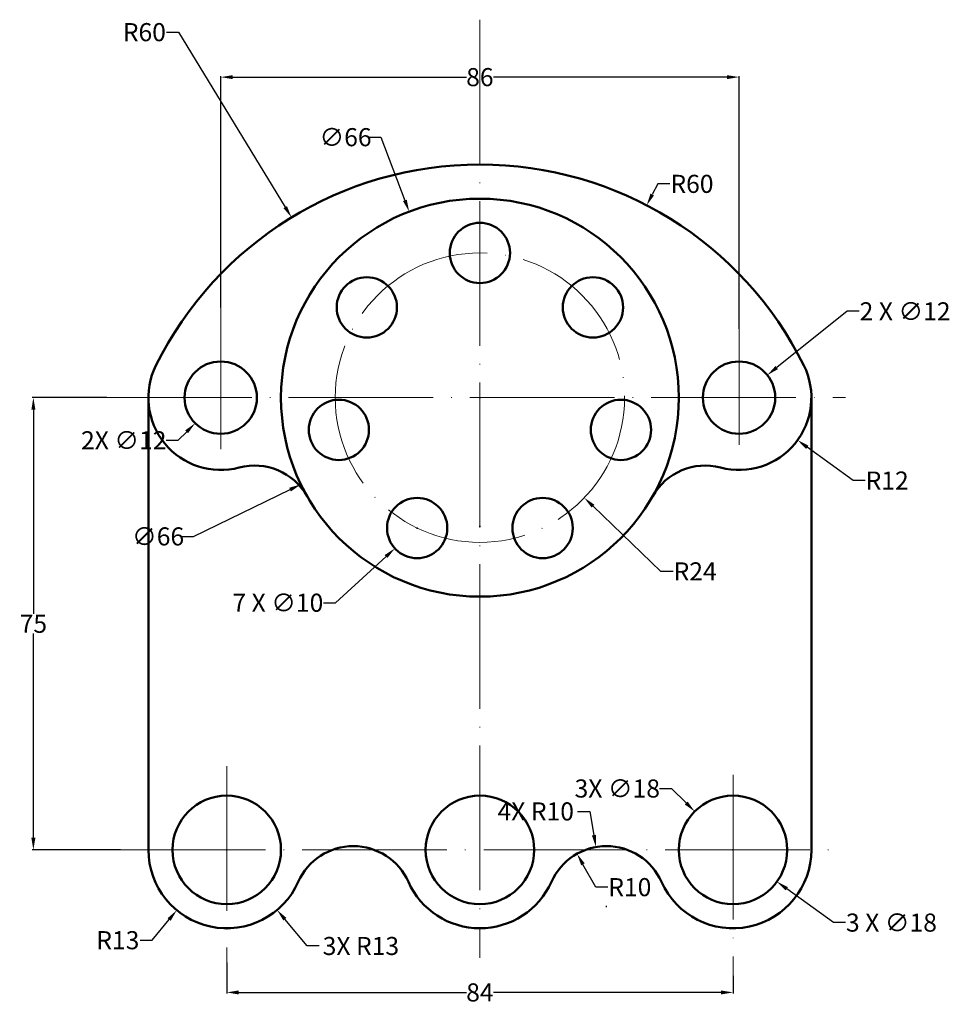
# Model space of a CAD drawing. Units: inches. Extents: x 328 to 483, y 163 to 326.
import ezdxf

# ---------------------------------------------------------------- set-up
doc = ezdxf.new("R2010")
doc.units = ezdxf.units.IN
doc.header["$MEASUREMENT"] = 0
doc.linetypes.add('ACAD_ISO04W100', pattern=[30, 24, -3, 0, -3])
for name, color, linetype, lineweight in [('M-CNTR', 4, 'ACAD_ISO04W100', 18), ('M-DIMS', 2, 'Continuous', 25), ('M-OUTL', 7, 'Continuous', 50)]:
    doc.layers.add(name, color=color, linetype=linetype, lineweight=lineweight)
doc.styles.get("Standard").update_dxf_attribs({"font": 'arial.ttf'})
doc.dimstyles.get("Standard").update_dxf_attribs({"dimtxt": 3, "dimasz": 2, "dimexe": 0.18, "dimexo": 0.0625, "dimgap": 0.09, "dimtad": 0, "dimtih": 1, "dimtoh": 1, "dimdec": 0, "dimzin": 0, "dimdsep": 46, "dimtxsty": 'Standard', "dimcen": 0.09, "dimclrd": 1, "dimclre": 1, "dimadec": 0, "dimazin": 0, "dimtfac": 1, "dimtdec": 0, "dimtofl": 0, "dimtmove": 0, "dimatfit": 3, "dimfxl": 1, "dimtolj": 1, "dimtzin": 0, "dimarcsym": 0})

# ---------------------------------------------------------------- blocks, each defined once
blk = doc.blocks.new('*U1')
blk.add_circle((0, 0), 5)
blk = doc.blocks.new('*U2')
at = {"layer": 'M-OUTL', "color": 0, "linetype": 'ByBlock', "lineweight": -2, "transparency": 16777216}
blk.add_blockref('*U1', (404.65, 287.76), dxfattribs=at)
for p, rotation in [((385.89, 278.73), 51.42857142857143), ((423.41, 278.73), 308.5714285714285), ((381.25, 258.42), 102.8571428571428), ((428.05, 258.42), 257.1428571428572), ((394.24, 242.14), 154.2857142857143), ((415.06, 242.14), 205.7142857142856)]:
    blk.add_blockref('*U1', p, dxfattribs=dict(at, rotation=rotation))
blk = doc.blocks.new('*D3')
at = {"layer": 'Defpoints', "color": 0, "transparency": 16777216}
for p in [(439.36, 194.04), (453.94, 183.49)]:
    blk.add_point(p, dxfattribs=at)
at = {"layer": 'M-DIMS', "color": 0, "lineweight": -2, "transparency": 16777216}
for p, q in [((446.56, 188.76), (446.74, 188.76)), ((446.65, 188.67), (446.65, 188.85)), ((463.34, 176.7), (455.57, 182.32)), ((465.34, 176.7), (463.34, 176.7))]:
    blk.add_line(p, q, dxfattribs=at)
at = {"layer": 'M-DIMS', "color": 0, "transparency": 16777216}
blk.add_solid([(455.76, 182.59), (455.37, 182.05), (453.94, 183.49)], dxfattribs=at)
at = {"layer": 'M-DIMS', "color": 0, "transparency": 16777216, "insert": (472.94, 176.7), "char_height": 3, "attachment_point": 5}
blk.add_mtext('\\A1;3 X ∅18', dxfattribs=at)
blk = doc.blocks.new('*D4')
at = {"layer": 'Defpoints', "color": 0, "transparency": 16777216}
for p in [(420.77, 188.11), (425.65, 179.38)]:
    blk.add_point(p, dxfattribs=at)
at = {"layer": 'M-DIMS', "color": 0, "lineweight": -2, "transparency": 16777216}
for p, q in [((423.87, 182.58), (421.75, 186.36)), ((425.87, 182.58), (423.87, 182.58))]:
    blk.add_line(p, q, dxfattribs=at)
at = {"layer": 'M-DIMS', "color": 0, "transparency": 16777216}
blk.add_solid([(422.04, 186.53), (421.46, 186.2), (420.77, 188.11)], dxfattribs=at)
at = {"layer": 'M-DIMS', "color": 0, "transparency": 16777216, "insert": (429.53, 182.58), "char_height": 3, "attachment_point": 5}
blk.add_mtext('\\A1;R10', dxfattribs=at)
blk = doc.blocks.new('*D5')
at = {"layer": 'Defpoints', "color": 0, "transparency": 16777216}
for p in [(362.65, 170.14), (446.65, 167.94), (446.65, 165.12)]:
    blk.add_point(p, dxfattribs=at)
at = {"layer": 'M-DIMS', "color": 0, "lineweight": -2, "transparency": 16777216}
for p, q in [((362.65, 170.08), (362.65, 164.94)), ((446.65, 167.88), (446.65, 164.94)), ((364.65, 165.12), (402.42, 165.12)), ((444.65, 165.12), (406.89, 165.12))]:
    blk.add_line(p, q, dxfattribs=at)
at = {"layer": 'M-DIMS', "color": 0, "transparency": 16777216}
for points in [[(364.65, 165.45), (364.65, 164.78), (362.65, 165.12)], [(444.65, 165.45), (444.65, 164.78), (446.65, 165.12)]]:
    blk.add_solid(points, dxfattribs=at)
at = {"layer": 'M-DIMS', "color": 0, "transparency": 16777216, "insert": (404.65, 165.12), "char_height": 3, "attachment_point": 5}
blk.add_mtext('\\A1;84', dxfattribs=at)
blk = doc.blocks.new('*D6')
at = {"layer": 'Defpoints', "color": 0, "transparency": 16777216}
for p in [(362.65, 188.76), (354.36, 178.75)]:
    blk.add_point(p, dxfattribs=at)
at = {"layer": 'M-DIMS', "color": 0, "lineweight": -2, "transparency": 16777216}
for p, q in [((362.56, 188.76), (362.74, 188.76)), ((362.65, 188.67), (362.65, 188.85)), ((350.26, 173.78), (353.09, 177.21)), ((348.26, 173.78), (350.26, 173.78))]:
    blk.add_line(p, q, dxfattribs=at)
at = {"layer": 'M-DIMS', "color": 0, "transparency": 16777216}
blk.add_solid([(352.83, 177.42), (353.34, 176.99), (354.36, 178.75)], dxfattribs=at)
at = {"layer": 'M-DIMS', "color": 0, "transparency": 16777216, "insert": (344.58, 173.78), "char_height": 3, "attachment_point": 5}
blk.add_mtext('\\A1;R13', dxfattribs=at)
blk = doc.blocks.new('*D7')
at = {"layer": 'Defpoints', "color": 0, "transparency": 16777216}
for p in [(342.79, 263.76), (330.56, 188.76), (345.08, 188.76)]:
    blk.add_point(p, dxfattribs=at)
at = {"layer": 'M-DIMS', "color": 0, "lineweight": -2, "transparency": 16777216}
for p, q in [((342.73, 263.76), (330.38, 263.76)), ((330.56, 261.76), (330.56, 227.88)), ((330.56, 190.76), (330.56, 224.65)), ((345.02, 188.76), (330.38, 188.76))]:
    blk.add_line(p, q, dxfattribs=at)
at = {"layer": 'M-DIMS', "color": 0, "transparency": 16777216}
for points in [[(330.23, 261.76), (330.9, 261.76), (330.56, 263.76)], [(330.23, 190.76), (330.9, 190.76), (330.56, 188.76)]]:
    blk.add_solid(points, dxfattribs=at)
at = {"layer": 'M-DIMS', "color": 0, "transparency": 16777216, "insert": (330.56, 226.26), "char_height": 3, "attachment_point": 5}
blk.add_mtext('\\A1;75', dxfattribs=at)
blk = doc.blocks.new('*D8')
at = {"layer": 'Defpoints', "color": 0, "transparency": 16777216}
for p in [(447.65, 263.76), (457.36, 256.71)]:
    blk.add_point(p, dxfattribs=at)
at = {"layer": 'M-DIMS', "color": 0, "lineweight": -2, "transparency": 16777216}
for p, q in [((447.56, 263.76), (447.74, 263.76)), ((447.65, 263.67), (447.65, 263.85)), ((466.57, 250.01), (458.97, 255.53)), ((468.57, 250.01), (466.57, 250.01))]:
    blk.add_line(p, q, dxfattribs=at)
at = {"layer": 'M-DIMS', "color": 0, "transparency": 16777216}
blk.add_solid([(459.17, 255.8), (458.78, 255.26), (457.36, 256.71)], dxfattribs=at)
at = {"layer": 'M-DIMS', "color": 0, "transparency": 16777216, "insert": (472.23, 250.01), "char_height": 3, "attachment_point": 5}
blk.add_mtext('\\A1;R12', dxfattribs=at)
blk = doc.blocks.new('*D9')
at = {"layer": 'Defpoints', "color": 0, "transparency": 16777216}
for p in [(404.65, 263.76), (421.97, 247.15)]:
    blk.add_point(p, dxfattribs=at)
at = {"layer": 'M-DIMS', "color": 0, "lineweight": -2, "transparency": 16777216}
for p, q in [((404.56, 263.76), (404.74, 263.76)), ((404.65, 263.67), (404.65, 263.85)), ((434.7, 234.95), (423.42, 245.77)), ((436.7, 234.95), (434.7, 234.95))]:
    blk.add_line(p, q, dxfattribs=at)
at = {"layer": 'M-DIMS', "color": 0, "transparency": 16777216}
blk.add_solid([(423.65, 246.01), (423.19, 245.53), (421.97, 247.15)], dxfattribs=at)
at = {"layer": 'M-DIMS', "color": 0, "transparency": 16777216, "insert": (440.37, 234.95), "char_height": 3, "attachment_point": 5}
blk.add_mtext('\\A1;R24', dxfattribs=at)
blk = doc.blocks.new('*D10')
at = {"layer": 'Defpoints', "color": 0, "transparency": 16777216}
for p in [(397.92, 245.52), (390.55, 238.76)]:
    blk.add_point(p, dxfattribs=at)
at = {"layer": 'M-DIMS', "color": 0, "lineweight": -2, "transparency": 16777216}
for p, q in [((394.15, 242.14), (394.33, 242.14)), ((394.24, 242.05), (394.24, 242.23)), ((380.71, 229.75), (389.08, 237.41)), ((378.71, 229.75), (380.71, 229.75))]:
    blk.add_line(p, q, dxfattribs=at)
at = {"layer": 'M-DIMS', "color": 0, "transparency": 16777216}
blk.add_solid([(388.85, 237.66), (389.3, 237.17), (390.55, 238.76)], dxfattribs=at)
at = {"layer": 'M-DIMS', "color": 0, "transparency": 16777216, "insert": (371.13, 229.75), "char_height": 3, "attachment_point": 5}
blk.add_mtext('\\A1;7 X ∅10', dxfattribs=at)
blk = doc.blocks.new('*D11')
at = {"layer": 'Defpoints', "color": 0, "transparency": 16777216}
for p in [(432.33, 295.67), (404.65, 242.43)]:
    blk.add_point(p, dxfattribs=at)
at = {"layer": 'M-DIMS', "color": 0, "lineweight": -2, "transparency": 16777216}
for p, q in [((434.17, 299.22), (433.25, 297.44)), ((436.17, 299.22), (434.17, 299.22)), ((404.56, 242.43), (404.74, 242.43)), ((404.65, 242.34), (404.65, 242.52))]:
    blk.add_line(p, q, dxfattribs=at)
at = {"layer": 'M-DIMS', "color": 0, "transparency": 16777216}
blk.add_solid([(432.95, 297.6), (433.54, 297.29), (432.33, 295.67)], dxfattribs=at)
at = {"layer": 'M-DIMS', "color": 0, "transparency": 16777216, "insert": (439.84, 299.22), "char_height": 3, "attachment_point": 5}
blk.add_mtext('\\A1;R60', dxfattribs=at)
blk = doc.blocks.new('*D12')
at = {"layer": 'Defpoints', "color": 0, "transparency": 16777216}
for p in [(447.65, 316.92), (361.65, 278.66), (447.65, 275.13)]:
    blk.add_point(p, dxfattribs=at)
at = {"layer": 'M-DIMS', "color": 0, "lineweight": -2, "transparency": 16777216}
for p, q in [((361.65, 278.72), (361.65, 317.1)), ((363.65, 316.92), (402.41, 316.92)), ((445.65, 316.92), (406.89, 316.92)), ((447.65, 275.19), (447.65, 317.1))]:
    blk.add_line(p, q, dxfattribs=at)
at = {"layer": 'M-DIMS', "color": 0, "transparency": 16777216}
for points in [[(363.65, 317.25), (363.65, 316.59), (361.65, 316.92)], [(445.65, 317.25), (445.65, 316.59), (447.65, 316.92)]]:
    blk.add_solid(points, dxfattribs=at)
at = {"layer": 'M-DIMS', "color": 0, "transparency": 16777216, "insert": (404.65, 316.92), "char_height": 3, "attachment_point": 5}
blk.add_mtext('\\A1;86', dxfattribs=at)
blk = doc.blocks.new('*D13')
at = {"layer": 'Defpoints', "color": 0, "transparency": 16777216}
for p in [(452.34, 267.5), (442.96, 260.02)]:
    blk.add_point(p, dxfattribs=at)
at = {"layer": 'M-DIMS', "color": 0, "lineweight": -2, "transparency": 16777216}
for p, q in [((465.59, 278.08), (453.9, 268.75)), ((467.59, 278.08), (465.59, 278.08)), ((447.56, 263.76), (447.74, 263.76)), ((447.65, 263.67), (447.65, 263.85))]:
    blk.add_line(p, q, dxfattribs=at)
at = {"layer": 'M-DIMS', "color": 0, "transparency": 16777216}
blk.add_solid([(453.7, 269.01), (454.11, 268.49), (452.34, 267.5)], dxfattribs=at)
at = {"layer": 'M-DIMS', "color": 0, "transparency": 16777216, "insert": (475.2, 278.08), "char_height": 3, "attachment_point": 5}
blk.add_mtext('\\A1;2 X ∅12', dxfattribs=at)
blk = doc.blocks.new('*D14')
at = {"layer": 'Defpoints', "color": 0, "transparency": 16777216}
for p in [(392.92, 294.61), (416.38, 232.92)]:
    blk.add_point(p, dxfattribs=at)
at = {"layer": 'M-DIMS', "color": 0, "lineweight": -2, "transparency": 16777216}
for p, q in [((386.23, 306.96), (388.23, 306.96)), ((388.23, 306.96), (392.21, 296.48)), ((404.56, 263.76), (404.74, 263.76)), ((404.65, 263.67), (404.65, 263.85))]:
    blk.add_line(p, q, dxfattribs=at)
at = {"layer": 'M-DIMS', "color": 0, "transparency": 16777216}
blk.add_solid([(392.52, 296.6), (391.9, 296.36), (392.92, 294.61)], dxfattribs=at)
at = {"layer": 'M-DIMS', "color": 0, "transparency": 16777216, "insert": (382.36, 306.96), "char_height": 3, "attachment_point": 5}
blk.add_mtext('\\A1;∅66', dxfattribs=at)
blk = doc.blocks.new('*D15')
at = {"layer": 'Defpoints', "color": 0, "transparency": 16777216}
for p in [(373.4, 293.65), (404.65, 242.43)]:
    blk.add_point(p, dxfattribs=at)
at = {"layer": 'M-DIMS', "color": 1, "lineweight": -2, "transparency": 16777216}
for p, q in [((352.65, 324.38), (354.65, 324.38)), ((354.65, 324.38), (372.36, 295.36)), ((404.56, 242.43), (404.74, 242.43)), ((404.65, 242.34), (404.65, 242.52))]:
    blk.add_line(p, q, dxfattribs=at)
at = {"layer": 'M-DIMS', "color": 1, "transparency": 16777216}
blk.add_solid([(372.64, 295.53), (372.07, 295.18), (373.4, 293.65)], dxfattribs=at)
at = {"layer": 'M-DIMS', "color": 0, "transparency": 16777216, "insert": (348.98, 324.38), "char_height": 3, "attachment_point": 5}
blk.add_mtext('\\A1;R60', dxfattribs=at)
blk = doc.blocks.new('*D16')
at = {"layer": 'Defpoints', "color": 0, "transparency": 16777216}
for p in [(434.35, 278.15), (374.95, 249.38)]:
    blk.add_point(p, dxfattribs=at)
at = {"layer": 'M-DIMS', "color": 1, "lineweight": -2, "transparency": 16777216}
for p, q in [((404.56, 263.76), (404.74, 263.76)), ((404.65, 263.67), (404.65, 263.85)), ((357.13, 240.75), (373.15, 248.51)), ((355.13, 240.75), (357.13, 240.75))]:
    blk.add_line(p, q, dxfattribs=at)
at = {"layer": 'M-DIMS', "color": 1, "transparency": 16777216}
blk.add_solid([(373.01, 248.81), (373.3, 248.21), (374.95, 249.38)], dxfattribs=at)
at = {"layer": 'M-DIMS', "color": 0, "transparency": 16777216, "insert": (351.26, 240.75), "char_height": 3, "attachment_point": 5}
blk.add_mtext('\\A1;∅66', dxfattribs=at)
blk = doc.blocks.new('*D17')
at = {"layer": 'Defpoints', "color": 0, "transparency": 16777216}
for p in [(365.89, 268.01), (357.41, 259.52)]:
    blk.add_point(p, dxfattribs=at)
at = {"layer": 'M-DIMS', "color": 1, "lineweight": -2, "transparency": 16777216}
for p, q in [((361.56, 263.76), (361.74, 263.76)), ((361.65, 263.67), (361.65, 263.85)), ((354.58, 256.69), (356, 258.1)), ((352.58, 256.69), (354.58, 256.69))]:
    blk.add_line(p, q, dxfattribs=at)
at = {"layer": 'M-DIMS', "color": 1, "transparency": 16777216}
blk.add_solid([(355.76, 258.34), (356.23, 257.87), (357.41, 259.52)], dxfattribs=at)
at = {"layer": 'M-DIMS', "color": 0, "transparency": 16777216, "insert": (345.56, 256.69), "char_height": 3, "attachment_point": 5}
blk.add_mtext('\\A1;2X ∅12', dxfattribs=at)
blk = doc.blocks.new('*D18')
at = {"layer": 'Defpoints', "color": 0, "transparency": 16777216}
for p in [(362.65, 188.76), (371, 178.8)]:
    blk.add_point(p, dxfattribs=at)
at = {"layer": 'M-DIMS', "color": 1, "lineweight": -2, "transparency": 16777216}
for p, q in [((362.56, 188.76), (362.74, 188.76)), ((362.65, 188.67), (362.65, 188.85)), ((376.01, 172.82), (372.29, 177.27)), ((378.01, 172.82), (376.01, 172.82))]:
    blk.add_line(p, q, dxfattribs=at)
at = {"layer": 'M-DIMS', "color": 1, "transparency": 16777216}
blk.add_solid([(372.54, 177.48), (372.03, 177.05), (371, 178.8)], dxfattribs=at)
at = {"layer": 'M-DIMS', "color": 0, "transparency": 16777216, "insert": (384.91, 172.82), "char_height": 3, "attachment_point": 5}
blk.add_mtext('\\A1;3X R13', dxfattribs=at)
blk = doc.blocks.new('*D19')
at = {"layer": 'Defpoints', "color": 0, "transparency": 16777216}
for p in [(423.91, 189.23), (425.65, 179.38)]:
    blk.add_point(p, dxfattribs=at)
at = {"layer": 'M-DIMS', "color": 1, "lineweight": -2, "transparency": 16777216}
for p, q in [((420.87, 195.14), (422.87, 195.14)), ((422.87, 195.14), (423.56, 191.2)), ((425.56, 179.38), (425.74, 179.38)), ((425.65, 179.29), (425.65, 179.47))]:
    blk.add_line(p, q, dxfattribs=at)
at = {"layer": 'M-DIMS', "color": 1, "transparency": 16777216}
blk.add_solid([(423.89, 191.26), (423.24, 191.14), (423.91, 189.23)], dxfattribs=at)
at = {"layer": 'M-DIMS', "color": 0, "transparency": 16777216, "insert": (413.92, 195.14), "char_height": 3, "attachment_point": 5}
blk.add_mtext('\\A1;4X R10', dxfattribs=at)
blk = doc.blocks.new('*D20')
at = {"layer": 'Defpoints', "color": 0, "transparency": 16777216}
for p in [(440.29, 195.13), (453.01, 182.4)]:
    blk.add_point(p, dxfattribs=at)
at = {"layer": 'M-DIMS', "color": 1, "lineweight": -2, "transparency": 16777216}
for p, q in [((434.47, 198.94), (436.47, 198.94)), ((436.47, 198.94), (438.87, 196.54)), ((446.56, 188.76), (446.74, 188.76)), ((446.65, 188.67), (446.65, 188.85))]:
    blk.add_line(p, q, dxfattribs=at)
at = {"layer": 'M-DIMS', "color": 1, "transparency": 16777216}
blk.add_solid([(439.11, 196.78), (438.64, 196.3), (440.29, 195.13)], dxfattribs=at)
at = {"layer": 'M-DIMS', "color": 0, "transparency": 16777216, "insert": (427.45, 198.94), "char_height": 3, "attachment_point": 5}
blk.add_mtext('\\A1;3X ∅18', dxfattribs=at)

msp = doc.modelspace()

# ---------------------------------------------------------------- linework, layer by layer
at = {"layer": 'M-CNTR'}
for p, q in [((404.65, 326.45), (404.65, 170.88)), ((361.65, 255.23), (361.65, 278.66)), ((447.65, 255.94), (447.65, 275.13)), ((342.79, 263.76), (465.33, 263.76)), ((362.65, 202.66), (362.65, 170.14)), ((446.65, 201.19), (446.65, 167.94)), ((345.08, 188.76), (464.95, 188.76))]:
    msp.add_line(p, q, dxfattribs=at)
msp.add_circle((404.65, 263.76), 24, dxfattribs=at)
at = {"layer": 'M-OUTL'}
for p, q in [((349.65, 188.76), (349.65, 263.76)), ((459.65, 188.76), (459.65, 263.76))]:
    msp.add_line(p, q, dxfattribs=at)
for centre, radius in [((404.65, 263.76), 33), ((361.65, 263.76), 6), ((447.65, 263.76), 6), ((362.65, 188.76), 9), ((404.65, 188.76), 9), ((446.65, 188.76), 9)]:
    msp.add_circle(centre, radius, dxfattribs=at)
for centre, radius, start, end in [((404.65, 242.43), 60, 26.3843, 153.6157), ((361.65, 263.76), 12, 153.6157, 284.8218), ((447.65, 263.76), 12, 255.1782, 26.3843), ((367.28, 242.49), 10, 29.6436, 104.8218), ((442.02, 242.49), 10, 75.1782, 150.3564), ((362.65, 188.76), 13, 180, 335.9294), ((383.65, 179.38), 10, 24.0706, 155.9294), ((425.65, 179.38), 10, 24.0706, 155.9294), ((446.65, 188.76), 13, 204.0706, 0), ((404.65, 188.76), 13, 204.0706, 335.9294)]:
    msp.add_arc(centre, radius, start, end, dxfattribs=at)

# ---------------------------------------------------------------- block references
msp.add_blockref('*U2', (0, 0), dxfattribs=at)

# ---------------------------------------------------------------- dimensions: what is measured, and where the dimension line sits
at = {"layer": 'M-DIMS'}
for center, mpoint, override, picture, middle in [((404.65, 242.43), (373.4, 293.65), {"dimdec": 0, "dimlfac": 1, "dimrnd": 0, "dimzin": 0, "dimdsep": 46, "dimlunit": 2}, '*D15', (348.98, 324.38)), ((404.65, 263.76), (421.97, 247.15), {"dimclrd": 0, "dimclre": 0, "dimclrt": 0}, '*D9', (440.37, 234.95)), ((447.65, 263.76), (457.36, 256.71), {"dimclrd": 0, "dimclre": 0, "dimclrt": 0}, '*D8', (472.23, 250.01)), ((362.65, 188.76), (354.36, 178.75), {"dimclrd": 0, "dimclre": 0, "dimclrt": 0}, '*D6', (344.58, 173.78)), ((425.65, 179.38), (420.77, 188.11), {"dimclrd": 0, "dimclre": 0, "dimclrt": 0}, '*D4', (429.53, 182.58))]:
    dim = msp.add_radius_dim(center=center, mpoint=mpoint, dimstyle='Standard', override=override, dxfattribs=at)
    dim.commit()
    dim.dimension.update_dxf_attribs({"geometry": picture, "text_midpoint": middle, "dimtype": 164})
for base, p1, p2, picture, middle in [((447.65, 316.92), (361.65, 278.66), (447.65, 275.13), '*D12', (404.65, 316.92)), ((446.65, 165.12), (362.65, 170.14), (446.65, 167.94), '*D5', (404.65, 165.12))]:
    dim = msp.add_linear_dim(base=base, p1=p1, p2=p2, dimstyle='Standard', override={"dimclrd": 0, "dimclre": 0, "dimclrt": 0}, dxfattribs=at)
    dim.commit()
    dim.dimension.update_dxf_attribs({"geometry": picture, "text_midpoint": middle})
for p1, p2, override, picture, middle in [((416.38, 232.92), (392.92, 294.61), {"dimclrd": 0, "dimclre": 0, "dimclrt": 0}, '*D14', (382.36, 306.96)), ((434.35, 278.15), (374.95, 249.38), {"dimdec": 0, "dimlfac": 1, "dimrnd": 0, "dimzin": 0, "dimdsep": 46, "dimlunit": 2}, '*D16', (351.26, 240.75))]:
    dim = msp.add_diameter_dim_2p(p1=p1, p2=p2, dimstyle='Standard', override=override, dxfattribs=at)
    dim.commit()
    dim.dimension.update_dxf_attribs({"geometry": picture, "text_midpoint": middle, "dimtype": 163})
dim = msp.add_radius_dim(center=(404.65, 242.43), mpoint=(432.33, 295.67), dimstyle='Standard', override={"dimclrd": 0, "dimclre": 0, "dimclrt": 0}, dxfattribs=at)
dim.commit()
dim.dimension.update_dxf_attribs({"geometry": '*D11', "text_midpoint": (439.84, 299.22)})
for p1, p2, text, override, picture, middle in [((442.96, 260.02), (452.34, 267.5), '2 X <>', {"dimclrd": 0, "dimclre": 0, "dimclrt": 0}, '*D13', (475.2, 278.08)), ((365.89, 268.01), (357.41, 259.52), '2X <>', {"dimdec": 0, "dimlfac": 1, "dimrnd": 0, "dimzin": 0, "dimdsep": 46, "dimlunit": 2}, '*D17', (345.56, 256.69)), ((397.92, 245.52), (390.55, 238.76), '7 X <>', {"dimclrd": 0, "dimclre": 0, "dimclrt": 0}, '*D10', (371.13, 229.75)), ((453.01, 182.4), (440.29, 195.13), '3X <>', {"dimdec": 0, "dimlfac": 1, "dimrnd": 0, "dimzin": 0, "dimdsep": 46, "dimlunit": 2}, '*D20', (427.45, 198.94)), ((439.36, 194.04), (453.94, 183.49), '3 X <>', {"dimclrd": 0, "dimclre": 0, "dimclrt": 0}, '*D3', (472.94, 176.7))]:
    dim = msp.add_diameter_dim_2p(p1=p1, p2=p2, text=text, dimstyle='Standard', override=override, dxfattribs=at)
    dim.commit()
    dim.dimension.update_dxf_attribs({"geometry": picture, "text_midpoint": middle, "dimtype": 163})
dim = msp.add_linear_dim(base=(330.56, 188.76), p1=(342.79, 263.76), p2=(345.08, 188.76), angle=90, dimstyle='Standard', override={"dimclrd": 0, "dimclre": 0, "dimclrt": 0}, dxfattribs=at)
dim.commit()
dim.dimension.update_dxf_attribs({"geometry": '*D7', "text_midpoint": (330.56, 226.26)})
for center, mpoint, text, picture, middle in [((425.65, 179.38), (423.91, 189.23), '4X <>', '*D19', (413.92, 195.14)), ((362.65, 188.76), (371, 178.8), '3X <>', '*D18', (384.91, 172.82))]:
    dim = msp.add_radius_dim(center=center, mpoint=mpoint, text=text, dimstyle='Standard', override={"dimdec": 0, "dimlfac": 1, "dimrnd": 0, "dimzin": 0, "dimdsep": 46, "dimlunit": 2}, dxfattribs=at)
    dim.commit()
    dim.dimension.update_dxf_attribs({"geometry": picture, "text_midpoint": middle, "dimtype": 164})

doc.saveas('drawing.dxf')
